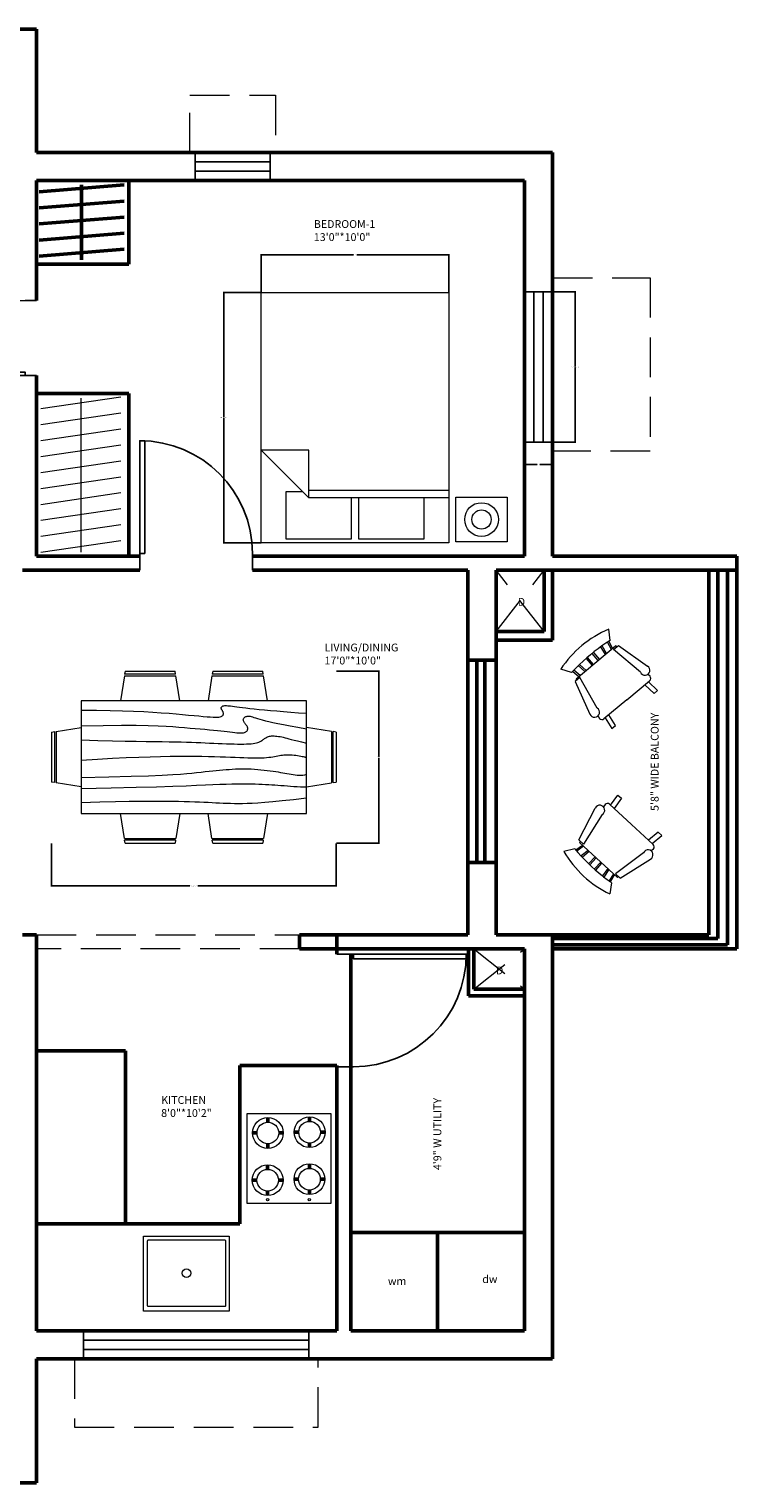
# Model space of a CAD drawing. Units: inches. Extents: x 291 to 2631, y 456 to 2623.
# Tile 19 of 22: x 2370 to 2596, y 1611 to 2076. Entities that reach past the tile are written whole.
import ezdxf

# ---------------------------------------------------------------- set-up
doc = ezdxf.new("R2010")
doc.units = ezdxf.units.IN
doc.linetypes.add('DASHED', pattern=[19.05, 12.7, -6.35])
for name, color, linetype, lineweight in [('A-ANNO-DIMS', 2, 'Continuous', 18), ('A-ANNO-TEXT', 3, 'Continuous', 25), ('A-AREA-IDEN', 7, 'Continuous', 25), ('A-DOOR', 3, 'Continuous', 25), ('A-FLOR-OVHD', 1, 'DASHED', 18), ('A-FURN', 8, 'Continuous', 18), ('A-GLAZ', 4, 'Continuous', 25), ('A-WALL', 7, 'Continuous', 50)]:
    doc.layers.add(name, color=color, linetype=linetype, lineweight=lineweight)
doc.styles.get("Standard").update_dxf_attribs({"font": 'arial.ttf'})
doc.dimstyles.get("Standard").update_dxf_attribs({"dimtxt": 0.18, "dimasz": 0.18, "dimexe": 0.18, "dimexo": 0.0625, "dimgap": 0.09, "dimtad": 0, "dimtih": 1, "dimtoh": 1, "dimdec": 4, "dimzin": 0, "dimdsep": 46, "dimtxsty": 'Standard', "dimcen": 0.09, "dimadec": 0, "dimazin": 0, "dimtfac": 1, "dimtdec": 4, "dimtofl": 0, "dimtmove": 0, "dimatfit": 3, "dimfxl": 1, "dimtolj": 1, "dimtzin": 0, "dimarcsym": 0})

# ---------------------------------------------------------------- blocks, each defined once
blk = doc.blocks.new('Bed - Queen')
for p, q in [((0, -80.00003), (0, 0)), ((0, 0), (59.99999, 0)), ((59.99999, 0), (59.99999, -80.00003)), ((7.99999, -1.2), (28.79998, -1.2)), ((7.99999, -14.4), (7.99999, -1.2)), ((28.79998, -1.2), (28.79998, -14.4)), ((31.19999, -1.2), (51.99999, -1.2)), ((31.19999, -14.4), (31.19999, -1.2)), ((51.99999, -1.2), (51.99999, -16.4)), ((0, -14.4), (44.8, -14.4)), ((44.8, -16.8), (0, -16.8)), ((59.99999, -29.6), (44.8, -14.4)), ((44.8, -14.4), (44.8, -29.6)), ((51.99999, -16.4), (46.79936, -16.4)), ((44.8, -29.6), (59.99999, -29.6)), ((59.99999, -80.00003), (0, -80.00003))]:
    blk.add_line(p, q)
blk = doc.blocks.new('Dining Set - 36 x 72 in.')
for p, q in [((-22.2343, 26.00059), (-23.4847, 17.99762)), ((-22.2304, 26), (-5.7608, 26)), ((-22, 27.5), (-22.1562, 26.50042)), ((-5.8416, 26.5), (-22.1534, 26.5)), ((-22, 27.5), (-6, 27.5)), ((-5.8437, 26.49966), (-6, 27.5)), ((-4.5152, 17.99762), (-5.7655, 25.99926)), ((5.7657, 26.00059), (4.5153, 17.99762)), ((5.7696, 26), (22.2392, 26)), ((6, 27.5), (5.8438, 26.50042)), ((22.1584, 26.5), (5.8466, 26.5)), ((6, 27.5), (22, 27.5)), ((22.1563, 26.49966), (22, 27.5)), ((23.4848, 17.99762), (22.2345, 25.99926)), ((36, 18), (-36, 18)), ((-36, 18), (-36, -18)), ((36, -18), (36, 18)), ((-44.0006, 8.23428), (-35.9976, 9.48474)), ((44.0006, 8.23428), (35.9976, 9.48474)), ((-45.5, 8), (-44.5004, 8.15617)), ((-45.5, 8), (-45.5, -8)), ((-44.5, -8.15843), (-44.5, 8.15338)), ((-44, 8.23041), (-44, -8.23915)), ((44, 8.23041), (44, -8.23915)), ((44.5, -8.15843), (44.5, 8.15338)), ((45.5, 8), (44.5005, 8.15617)), ((45.5, 8), (45.5, -8)), ((-44.4997, -8.15631), (-45.5, -8)), ((-35.9976, -9.48476), (-43.9993, -8.2345)), ((35.9976, -9.48476), (43.9993, -8.2345)), ((44.4997, -8.15631), (45.5, -8)), ((-36, -18), (36, -18)), ((-22.2343, -26.0006), (-23.4847, -17.99762)), ((-4.5152, -17.99762), (-5.7655, -25.99928)), ((5.7657, -26.0006), (4.5153, -17.99762)), ((23.4848, -17.99762), (22.2345, -25.99928)), ((-22.2304, -26), (-5.7608, -26)), ((-22, -27.5), (-22.1562, -26.50044)), ((-5.8416, -26.5), (-22.1534, -26.5)), ((-22, -27.5), (-6, -27.5)), ((-5.8437, -26.49967), (-6, -27.5)), ((5.7696, -26), (22.2392, -26)), ((6, -27.5), (5.8438, -26.50044)), ((22.1584, -26.5), (5.8466, -26.5)), ((6, -27.5), (22, -27.5)), ((22.1563, -26.49967), (22, -27.5))]:
    blk.add_line(p, q)
for points in [[(-36, 15), (-31.1772, 14.97754), (-26.8079, 14.91406), (-22.8538, 14.81543), (-19.276, 14.6875), (-16.0362, 14.53613), (-13.0957, 14.36718), (-10.4159, 14.18652), (-7.9583, 14), (-5.6904, 13.81315), (-3.6035, 13.63021), (-1.6954, 13.45508), (0.0365, 13.29166), (1.5945, 13.14388), (2.9811, 13.01562), (4.1988, 12.9108), (5.25, 12.83333), (6.1393, 12.78613), (6.8802, 12.76823), (7.4883, 12.77767), (7.9792, 12.8125), (8.3685, 12.87077), (8.6719, 12.95052), (8.9049, 13.0498), (9.0833, 13.16666), (9.2205, 13.29899), (9.3216, 13.44401), (9.3895, 13.59879), (9.4271, 13.76041), (9.4373, 13.92594), (9.4232, 14.09245), (9.3875, 14.257), (9.3333, 14.41666), (9.2638, 14.56917), (9.1836, 14.71484), (9.0975, 14.85465), (9.0104, 14.98958), (8.9272, 15.1206), (8.8529, 15.2487), (8.7922, 15.37483), (8.75, 15.5), (8.7305, 15.62467), (8.7344, 15.74739), (8.7617, 15.86621), (8.8125, 15.97916), (8.8867, 16.08431), (8.9844, 16.17968), (9.1055, 16.26334), (9.25, 16.33333), (9.4189, 16.38802), (9.6172, 16.42708), (9.8506, 16.45052), (10.125, 16.45833), (10.4463, 16.45052), (10.8203, 16.42708), (11.2529, 16.38802), (11.75, 16.33333), (12.3184, 16.26318), (12.9694, 16.17838), (13.7151, 16.07991), (14.5677, 15.96875), (15.5395, 15.84586), (16.6426, 15.71224), (17.8893, 15.56884), (19.2917, 15.41666), (20.859, 15.25667), (22.5879, 15.08984), (24.4721, 14.91715), (26.5052, 14.73958), (28.6809, 14.5581), (30.9929, 14.3737), (33.4347, 14.18733), (36, 14)], [(-36, 10), (-28.9766, 10.14274), (-23.1725, 10.20442), (-18.4241, 10.19775), (-14.5677, 10.13541), (-11.4399, 10.03011), (-8.877, 9.89453), (-6.7154, 9.74137), (-4.7917, 9.58333), (-2.9698, 9.43082), (-1.2246, 9.28515), (0.4415, 9.14534), (2.026, 9.01041), (3.5266, 8.87939), (4.9408, 8.7513), (6.266, 8.62516), (7.5, 8.5), (8.6411, 8.37549), (9.6914, 8.2539), (10.6538, 8.13818), (11.5312, 8.03125), (12.3267, 7.93603), (13.043, 7.85547), (13.6831, 7.79248), (14.25, 7.75), (14.7471, 7.7303), (15.1797, 7.73307), (15.5537, 7.75732), (15.875, 7.80208), (16.1494, 7.86637), (16.3828, 7.94922), (16.5811, 8.04964), (16.75, 8.16666), (16.8944, 8.29915), (17.0143, 8.44531), (17.1089, 8.60319), (17.1771, 8.77083), (17.218, 8.94629), (17.2305, 9.1276), (17.2137, 9.31282), (17.1667, 9.5), (17.0895, 9.6875), (16.987, 9.875), (16.8649, 10.0625), (16.7292, 10.25), (16.5856, 10.4375), (16.4401, 10.625), (16.2985, 10.8125), (16.1667, 11), (16.05, 11.18733), (15.9518, 11.3737), (15.8752, 11.5581), (15.8229, 11.73958), (15.798, 11.91715), (15.8034, 12.08984), (15.842, 12.25667), (15.9167, 12.41666), (16.0295, 12.56836), (16.1784, 12.70833), (16.3605, 12.83268), (16.5729, 12.9375), (16.8127, 13.01888), (17.0768, 13.07291), (17.3625, 13.0957), (17.6667, 13.08333), (17.9894, 13.03312), (18.3418, 12.94726), (18.7382, 12.82918), (19.1927, 12.68229), (19.7195, 12.51001), (20.3327, 12.31575), (21.0465, 12.10294), (21.875, 11.875), (22.8357, 11.63354), (23.959, 11.37304), (25.2786, 11.08618), (26.8282, 10.76562), (28.6414, 10.40405), (30.752, 9.99414), (33.1936, 9.52856), (36, 9)], [(-36, 5.5), (-30.7157, 5.3348), (-26.069, 5.20963), (-21.9946, 5.11767), (-18.4271, 5.05208), (-15.3009, 5.00602), (-12.5508, 4.97265), (-10.1112, 4.94515), (-7.9167, 4.91666), (-5.909, 4.88167), (-4.0586, 4.83984), (-2.3429, 4.79215), (-0.7396, 4.73958), (0.7739, 4.6831), (2.22, 4.6237), (3.6213, 4.56233), (5, 4.5), (6.373, 4.43782), (7.7344, 4.3776), (9.0723, 4.32129), (10.375, 4.27083), (11.6309, 4.22819), (12.8281, 4.19531), (13.9551, 4.17415), (15, 4.16666), (15.954, 4.17448), (16.819, 4.19791), (17.6001, 4.23698), (18.3021, 4.29166), (18.9299, 4.36198), (19.4883, 4.44791), (19.9823, 4.54948), (20.4167, 4.66666), (20.7969, 4.79899), (21.1302, 4.94401), (21.4245, 5.09879), (21.6875, 5.26041), (21.9271, 5.42594), (22.1511, 5.59245), (22.3672, 5.757), (22.5834, 5.91666), (22.8065, 6.06868), (23.0404, 6.21093), (23.2879, 6.34147), (23.5521, 6.45833), (23.8358, 6.55957), (24.142, 6.64323), (24.4735, 6.70735), (24.8334, 6.75), (25.2235, 6.76969), (25.642, 6.76692), (26.0858, 6.74267), (26.5521, 6.69791), (27.0379, 6.63362), (27.5404, 6.55078), (28.0565, 6.45036), (28.5834, 6.33333), (29.1242, 6.19987), (29.7071, 6.04687), (30.3661, 5.87044), (31.1354, 5.66666), (32.0493, 5.43164), (33.142, 5.16146), (34.4475, 4.85221), (36, 4.5)], [(-36, -1), (-30.7915, -0.6591), (-26.0195, -0.38216), (-21.6519, -0.16284), (-17.6563, 0.00521), (-14.0005, 0.12833), (-10.6523, 0.21289), (-7.5796, 0.26522), (-4.75, 0.29166), (-2.134, 0.29793), (0.2878, 0.28711), (2.5317, 0.26163), (4.6146, 0.22396), (6.5529, 0.17651), (8.3633, 0.12174), (10.0623, 0.06209), (11.6667, 0), (13.1899, -0.06201), (14.6341, -0.1211), (15.9982, -0.17432), (17.2813, -0.21875), (18.4823, -0.25147), (19.6003, -0.26953), (20.6343, -0.27002), (21.5834, -0.25), (22.4481, -0.20768), (23.2357, -0.14584), (23.9549, -0.06836), (24.6146, 0.02083), (25.2235, 0.11784), (25.7904, 0.21875), (26.3241, 0.31966), (26.8334, 0.41666), (27.3265, 0.50618), (27.8099, 0.58593), (28.2894, 0.65397), (28.7709, 0.70833), (29.2601, 0.74707), (29.763, 0.76823), (30.2855, 0.76985), (30.8334, 0.75), (31.4088, 0.70784), (31.9994, 0.64713), (32.589, 0.57275), (33.1615, 0.48958), (33.7008, 0.4025), (34.1908, 0.3164), (34.6153, 0.23616), (34.9584, 0.16666), (35.2099, 0.11165), (35.3848, 0.07031), (35.504, 0.04069), (35.5886, 0.02083), (35.6594, 0.00879), (35.7377, 0.0026), (35.8442, 0.00032), (36, 0)], [(-36, -6.5), (-27.1843, -6.31267), (-20.084, -6.1263), (-14.469, -5.9419), (-10.1094, -5.76042), (-6.7752, -5.58285), (-4.2363, -5.41016), (-2.2629, -5.24333), (-0.625, -5.08334), (0.8708, -4.93099), (2.2715, -4.78646), (3.5872, -4.64974), (4.8281, -4.52084), (6.0046, -4.39974), (7.127, -4.28646), (8.2053, -4.18099), (9.25, -4.08334), (10.2705, -3.99382), (11.2734, -3.91407), (12.2647, -3.84603), (13.25, -3.79167), (14.2354, -3.75293), (15.2266, -3.73177), (16.2295, -3.73015), (17.25, -3.75), (18.2912, -3.79248), (19.3451, -3.85547), (20.4009, -3.93604), (21.4479, -4.03125), (22.4754, -4.13819), (23.4727, -4.25391), (24.4289, -4.37549), (25.3334, -4.5), (26.1785, -4.62492), (26.9694, -4.74935), (27.7145, -4.87281), (28.4219, -4.99479), (29.1, -5.11483), (29.7572, -5.23242), (30.4016, -5.34709), (31.0417, -5.45834), (31.6837, -5.56437), (32.3262, -5.65821), (32.9658, -5.73153), (33.599, -5.77604), (34.2224, -5.78345), (34.8327, -5.74545), (35.4264, -5.65373), (36, -5.5)], [(-36, -10), (-26.4022, -9.81299), (-18.4675, -9.62891), (-11.9839, -9.45069), (-6.7396, -9.28125), (-2.5226, -9.12354), (0.8789, -8.98047), (3.6769, -8.85498), (6.0833, -8.75), (8.2767, -8.66765), (10.3021, -8.60677), (12.1712, -8.56543), (13.8958, -8.54167), (15.4876, -8.53353), (16.9583, -8.53907), (18.3197, -8.55632), (19.5834, -8.58334), (20.7616, -8.61841), (21.8685, -8.66081), (22.9188, -8.71004), (23.9271, -8.76563), (24.9081, -8.82707), (25.8763, -8.89388), (26.8465, -8.96558), (27.8334, -9.04167), (28.8474, -9.12118), (29.8828, -9.20117), (30.93, -9.27824), (31.9792, -9.34896), (33.0205, -9.40991), (34.0443, -9.45768), (35.0407, -9.48885), (36, -9.5)], [(-36, -14.5), (-30.0881, -14.33513), (-25.0332, -14.21224), (-20.7312, -14.12647), (-17.0781, -14.07292), (-13.97, -14.04671), (-11.3027, -14.04297), (-8.9724, -14.05681), (-6.875, -14.08334), (-4.9224, -14.11833), (-3.0905, -14.16016), (-1.3709, -14.20785), (0.2448, -14.26042), (1.7647, -14.3169), (3.1973, -14.3763), (4.5507, -14.43767), (5.8333, -14.5), (7.0554, -14.5621), (8.235, -14.62175), (9.3922, -14.67652), (10.5469, -14.72396), (11.7192, -14.76164), (12.929, -14.78711), (14.1965, -14.79794), (15.5417, -14.79167), (16.9933, -14.76424), (18.6152, -14.70508), (20.4804, -14.60197), (22.6615, -14.44271), (25.2312, -14.21509), (28.2624, -13.9069), (31.8277, -13.50594), (36, -13)]]:
    blk.add_lwpolyline(points)
blk = doc.blocks.new('Chair - Rocking')
for p, q in [((-8, -4.5), (-10, -1.5)), ((-7.5, -4.5), (-7, -7)), ((-6.5, -7), (-7.02225, -4.43)), ((-4.5, -7), (-4.96674, -4.19951)), ((-4, -7), (-4.40532, -4.16272)), ((-1.5, -4.05012), (-1.5, -7)), ((-1, -7), (-1, -4.05012)), ((1, -7), (1, -4.04655)), ((1.5, -4.05012), (1.5, -7)), ((4, -7), (4.40187, -4.18694)), ((4.5, -7), (4.96761, -4.19437)), ((6.5, -7), (7, -4.4057)), ((7.5, -4.5), (7, -7)), ((8, -4.5), (10, -1.5)), ((-9, -7.5), (-12, -18.49999)), ((-7, -7.5), (-9, -7.5)), ((-9, -18.49999), (-7, -7.5)), ((-8.23428, -6.99939), (-8.3093, -7.47958)), ((-8.23041, -7), (8.23915, -7)), ((7, -7.5), (9, -7.5)), ((9, -18.49999), (7, -7.5)), ((8.31071, -7.48854), (8.23449, -7.00073)), ((9, -7.5), (12, -18.49999)), ((-10.36644, -20.64523), (-10.5, -21.49999)), ((-9, -22.49999), (-9.5, -26.49999)), ((0, -22.49999), (-9.5, -22.49999)), ((-8, -26.49999), (-7.5, -22.49999)), ((0, -22.49999), (9.5, -22.49999)), ((8, -26.49999), (7.5, -22.49999)), ((9, -22.49999), (9.5, -26.49999)), ((10.5, -21.49999), (10.3575, -20.58798)), ((-9.5, -26.49999), (-8, -26.49999)), ((9.5, -26.49999), (8, -26.49999))]:
    blk.add_line(p, q)
for centre, radius, start, end in [((0, -34.08333), 34.08333, 72.93847, 107.0615), ((0, -68.25004), 64.25, 93.92211, 97.15267), ((0, -68.25004), 64.25, 82.84733, 93.92211), ((-10.5, -18.99999), 1.58114, 161.5651, 18.43495), ((10.5, -18.99999), 1.58114, 161.5651, 18.43495), ((-9.5, -21.49999), 1, 180, 270), ((9.5, -21.49999), 1, 270, 0)]:
    blk.add_arc(centre, radius, start, end)
blk = doc.blocks.new('*U2')
for p, q in [((0, 0), (0, -6)), ((40, 0), (40, -6))]:
    blk.add_line(p, q)
blk.add_lwpolyline([(0, 0), (0, 40), (1.75, 40), (1.75, 0)], close=True)
blk.add_arc((0, 0), 40, 0, 90)
blk = doc.blocks.new('WIN-1800')
for p, q in [((0, 9), (72, 9)), ((0, 0), (0, 9)), ((0, 6), (72, 6)), ((72, 9), (72, 0)), ((72, 3), (0, 3)), ((72, 0), (0, 0))]:
    blk.add_line(p, q)
blk = doc.blocks.new('WIN-1200')
for p, q in [((0, 0), (0, 48)), ((0, 48), (9, 48)), ((3, 0), (3, 48)), ((6, 48), (6, 0)), ((9, 48), (9, 0)), ((9, 0), (0, 0))]:
    blk.add_line(p, q)
blk = doc.blocks.new('WIN-600')
for p, q in [((24, 9), (0, 9)), ((0, 9), (0, 0)), ((24, 6), (0, 6)), ((24, 0), (24, 9)), ((0, 3), (24, 3)), ((0, 0), (24, 0))]:
    blk.add_line(p, q)
blk = doc.blocks.new('*D24')
at = {"layer": 'A-ANNO-DIMS', "color": 0, "lineweight": -2, "transparency": 16777216}
for p, q in [((2537.27, 1991.61), (2544.59, 1991.61)), ((2544.41, 1991.43), (2544.41, 1967.79)), ((2544.41, 1943.79), (2544.41, 1967.43)), ((2537.27, 1943.61), (2544.59, 1943.61))]:
    blk.add_line(p, q, dxfattribs=at)
at = {"layer": 'A-ANNO-DIMS', "color": 0, "transparency": 16777216}
for points in [[(2544.38, 1991.43), (2544.44, 1991.43), (2544.41, 1991.61)], [(2544.38, 1943.79), (2544.44, 1943.79), (2544.41, 1943.61)]]:
    blk.add_solid(points, dxfattribs=at)
at = {"layer": 'DEFPOINTS', "color": 0, "transparency": 16777216}
for p in [(2537.21, 1991.61), (2544.41, 1991.61), (2537.21, 1943.61)]:
    blk.add_point(p, dxfattribs=at)
at = {"layer": 'A-ANNO-DIMS', "color": 0, "transparency": 16777216, "insert": (2544.41, 1967.61), "char_height": 0.18, "attachment_point": 5}
blk.add_mtext('\\A1;WINDOW W1200 48 TYP.', dxfattribs=at)
blk = doc.blocks.new('*D25')
at = {"layer": 'A-ANNO-DIMS', "color": 0, "lineweight": -2, "transparency": 16777216}
for p, q in [((2528.21, 1943.55), (2528.21, 1936.23)), ((2537.21, 1943.55), (2537.21, 1936.23)), ((2528.39, 1936.41), (2532.25, 1936.41)), ((2537.03, 1936.41), (2533.16, 1936.41))]:
    blk.add_line(p, q, dxfattribs=at)
at = {"layer": 'A-ANNO-DIMS', "color": 0, "transparency": 16777216}
for points in [[(2528.39, 1936.44), (2528.39, 1936.38), (2528.21, 1936.41)], [(2537.03, 1936.44), (2537.03, 1936.38), (2537.21, 1936.41)]]:
    blk.add_solid(points, dxfattribs=at)
at = {"layer": 'DEFPOINTS', "color": 0, "transparency": 16777216}
for p in [(2528.21, 1943.61), (2537.21, 1943.61), (2537.21, 1936.41)]:
    blk.add_point(p, dxfattribs=at)
at = {"layer": 'A-ANNO-DIMS', "color": 0, "transparency": 16777216, "insert": (2532.71, 1936.41), "char_height": 0.18, "attachment_point": 5}
blk.add_mtext('\\A1;9 TYP.', dxfattribs=at)
blk = doc.blocks.new('*D28')
at = {"layer": 'A-ANNO-DIMS', "color": 0, "lineweight": -2, "transparency": 16777216}
for p, q in [((2443.99, 1991.43), (2431.88, 1991.43)), ((2432.06, 1991.25), (2432.06, 1951.62)), ((2432.06, 1911.61), (2432.06, 1951.24)), ((2443.99, 1911.43), (2431.88, 1911.43))]:
    blk.add_line(p, q, dxfattribs=at)
at = {"layer": 'A-ANNO-DIMS', "color": 0, "transparency": 16777216}
for points in [[(2432.03, 1991.25), (2432.09, 1991.25), (2432.06, 1991.43)], [(2432.03, 1911.61), (2432.09, 1911.61), (2432.06, 1911.43)]]:
    blk.add_solid(points, dxfattribs=at)
at = {"layer": 'DEFPOINTS', "color": 0, "transparency": 16777216}
for p in [(2444.06, 1991.43), (2432.06, 1911.43), (2444.06, 1911.43)]:
    blk.add_point(p, dxfattribs=at)
at = {"layer": 'A-ANNO-DIMS', "color": 0, "transparency": 16777216, "insert": (2432.06, 1951.43), "char_height": 0.18, "attachment_point": 5}
blk.add_mtext('\\A1;QUEEN BED 80 TYP.', dxfattribs=at)
blk = doc.blocks.new('*D29')
at = {"layer": 'A-ANNO-DIMS', "color": 0, "lineweight": -2, "transparency": 16777216}
for p, q in [((2444.06, 1991.49), (2444.06, 2003.61)), ((2444.24, 2003.43), (2473.53, 2003.43)), ((2503.88, 2003.43), (2474.58, 2003.43)), ((2504.06, 1991.49), (2504.06, 2003.61))]:
    blk.add_line(p, q, dxfattribs=at)
at = {"layer": 'A-ANNO-DIMS', "color": 0, "transparency": 16777216}
for points in [[(2444.24, 2003.46), (2444.24, 2003.4), (2444.06, 2003.43)], [(2503.88, 2003.46), (2503.88, 2003.4), (2504.06, 2003.43)]]:
    blk.add_solid(points, dxfattribs=at)
at = {"layer": 'DEFPOINTS', "color": 0, "transparency": 16777216}
for p in [(2444.06, 2003.43), (2444.06, 1991.43), (2504.06, 1991.43)]:
    blk.add_point(p, dxfattribs=at)
at = {"layer": 'A-ANNO-DIMS', "color": 0, "transparency": 16777216, "insert": (2474.06, 2003.43), "char_height": 0.18, "attachment_point": 5}
blk.add_mtext('\\A1;60 TYP.', dxfattribs=at)
blk = doc.blocks.new('*D46')
at = {"layer": 'A-ANNO-DIMS', "color": 0, "lineweight": -2, "transparency": 16777216}
for p, q in [((2377.04, 1815.38), (2377.04, 1801.62)), ((2468.04, 1815.38), (2468.04, 1801.62)), ((2377.22, 1801.8), (2421.26, 1801.8)), ((2467.86, 1801.8), (2423.82, 1801.8))]:
    blk.add_line(p, q, dxfattribs=at)
at = {"layer": 'A-ANNO-DIMS', "color": 0, "transparency": 16777216}
for points in [[(2377.22, 1801.83), (2377.22, 1801.77), (2377.04, 1801.8)], [(2467.86, 1801.83), (2467.86, 1801.77), (2468.04, 1801.8)]]:
    blk.add_solid(points, dxfattribs=at)
at = {"layer": 'DEFPOINTS', "color": 0, "transparency": 16777216}
for p in [(2377.04, 1815.45), (2468.04, 1815.45), (2468.04, 1801.8)]:
    blk.add_point(p, dxfattribs=at)
at = {"layer": 'A-ANNO-DIMS', "color": 0, "transparency": 16777216, "insert": (2422.54, 1801.8), "char_height": 0.18, "attachment_point": 5}
blk.add_mtext('\\A1;DINING SET 91 TYP.', dxfattribs=at)
blk = doc.blocks.new('*D47')
at = {"layer": 'A-ANNO-DIMS', "color": 0, "lineweight": -2, "transparency": 16777216}
for p, q in [((2468.1, 1870.45), (2481.87, 1870.45)), ((2481.69, 1870.27), (2481.69, 1843.13)), ((2481.69, 1815.63), (2481.69, 1842.77)), ((2468.1, 1815.45), (2481.87, 1815.45))]:
    blk.add_line(p, q, dxfattribs=at)
at = {"layer": 'A-ANNO-DIMS', "color": 0, "transparency": 16777216}
for points in [[(2481.66, 1870.27), (2481.72, 1870.27), (2481.69, 1870.45)], [(2481.66, 1815.63), (2481.72, 1815.63), (2481.69, 1815.45)]]:
    blk.add_solid(points, dxfattribs=at)
at = {"layer": 'DEFPOINTS', "color": 0, "transparency": 16777216}
for p in [(2468.04, 1870.45), (2481.69, 1870.45), (2468.04, 1815.45)]:
    blk.add_point(p, dxfattribs=at)
at = {"layer": 'A-ANNO-DIMS', "color": 0, "transparency": 16777216, "insert": (2481.69, 1842.95), "char_height": 0.18, "attachment_point": 5}
blk.add_mtext('\\A1;55 TYP.', dxfattribs=at)

msp = doc.modelspace()

# ---------------------------------------------------------------- linework, layer by layer
at = {"layer": 'A-FLOR-OVHD'}
for p, q in [((2421.24, 2036.14), (2421.24, 2054.42)), ((2421.24, 2054.42), (2448.64, 2054.42)), ((2448.64, 2054.42), (2448.64, 2036.14)), ((2537.21, 1996.12), (2568.43, 1996.12)), ((2568.43, 1996.12), (2568.43, 1940.67)), ((2568.43, 1940.67), (2537.21, 1940.67)), ((2519.14, 1883.06), (2534.51, 1902.64)), ((2534.51, 1883.06), (2519.14, 1902.64)), ((2372.21, 1786.14), (2456.28, 1786.14)), ((2456.28, 1781.64), (2372.21, 1781.64)), ((2512, 1781.64), (2528.21, 1768.81)), ((2512, 1768.81), (2528.21, 1781.64)), ((2384.4, 1650.64), (2384.4, 1628.9)), ((2462.3, 1628.9), (2462.3, 1650.64)), ((2384.4, 1628.9), (2462.3, 1628.9))]:
    msp.add_line(p, q, dxfattribs=at)
at = {"layer": 'A-FURN'}
for p, q in [((2373.6, 1954.3), (2399.2, 1958.03)), ((2386.4, 1957.68), (2386.4, 1908.48)), ((2373.6, 1949.2), (2399.2, 1952.94)), ((2373.6, 1944.1), (2399.2, 1947.84)), ((2373.6, 1939.01), (2399.2, 1942.74)), ((2373.6, 1933.91), (2399.2, 1937.64)), ((2373.6, 1928.81), (2399.2, 1932.54)), ((2373.6, 1923.71), (2399.2, 1927.45)), ((2373.6, 1918.61), (2399.2, 1922.35)), ((2373.6, 1913.52), (2399.2, 1917.25)), ((2373.6, 1908.42), (2399.2, 1912.15))]:
    msp.add_line(p, q, dxfattribs=at)
for points in [[(2506.25, 1926.01), (2522.73, 1926.01), (2522.73, 1911.71), (2506.25, 1911.71)], [(2439.58, 1729.09), (2466.29, 1729.09), (2466.29, 1700.32), (2439.58, 1700.32)], [(2406.4, 1689.84), (2433.84, 1689.84), (2433.84, 1665.94), (2406.4, 1665.94)]]:
    msp.add_lwpolyline(points, close=True, dxfattribs=at)
msp.add_lwpolyline([(2408.04, 1688.73), (2432.34, 1688.73, -0.414214), (2432.64, 1688.43), (2432.64, 1667.66, -0.414214), (2432.34, 1667.36), (2408.04, 1667.36, -0.414214), (2407.74, 1667.66), (2407.74, 1688.43, -0.414214)], format="xyb", close=True, dxfattribs=at)
for centre, radius in [((2514.49, 1918.86), 5.39), ((2514.49, 1918.86), 3.08), ((2446.18, 1722.85), 4.92), ((2446.18, 1722.85), 3.46), ((2459.53, 1723.1), 4.92), ((2459.53, 1723.1), 3.46), ((2446.12, 1707.77), 4.92), ((2446.12, 1707.77), 3.46), ((2459.47, 1708.09), 4.92), ((2459.47, 1708.09), 3.46), ((2446.08, 1701.54), 0.363), ((2459.43, 1701.55), 0.363), ((2420.19, 1678.04), 1.36)]:
    msp.add_circle(centre, radius, dxfattribs=at)
at = {"layer": 'A-WALL'}
for p, q in [((2303.21, 2075.57), (2372.21, 2075.57)), ((2372.21, 2075.57), (2372.21, 2036.14)), ((2372.21, 2036.14), (2521.26, 2036.14)), ((2537.21, 2036.14), (2521.26, 2036.14)), ((2537.21, 2027.14), (2537.21, 2036.14)), ((2372.21, 2027.14), (2372.21, 1988.89)), ((2372.21, 2027.14), (2372.21, 1988.89)), ((2372.21, 2027.14), (2521.26, 2027.14)), ((2373.04, 2023.54), (2400.26, 2025.76)), ((2386.65, 2025.83), (2386.65, 2001.89)), ((2401.79, 2000.49), (2401.79, 2027.14)), ((2521.26, 2027.14), (2528.21, 2027.14)), ((2528.21, 2027.14), (2528.21, 1907.14)), ((2537.21, 2027.14), (2537.21, 1907.14)), ((2373.04, 2018.42), (2400.26, 2020.64)), ((2373.04, 2013.3), (2400.26, 2015.52)), ((2373.04, 2008.17), (2400.26, 2010.39)), ((2373.04, 2003.05), (2400.26, 2005.27)), ((2372.21, 2000.49), (2401.79, 2000.49)), ((2372.21, 1964.89), (2372.21, 1907.14)), ((2372.21, 1964.89), (2372.21, 1907.14)), ((2372.21, 1959.17), (2401.79, 1959.17)), ((2401.79, 1959.17), (2401.79, 1907.14)), ((2372.21, 1907.14), (2405.25, 1907.14)), ((2441.25, 1907.14), (2528.21, 1907.14)), ((2537.21, 1907.14), (2596.14, 1907.14)), ((2596.14, 1907.14), (2596.14, 1781.64)), ((2367.71, 1902.64), (2405.25, 1902.64)), ((2441.25, 1902.64), (2510.14, 1902.64)), ((2510.14, 1902.64), (2510.14, 1786.14)), ((2519.14, 1902.64), (2519.14, 1786.14)), ((2519.14, 1902.64), (2537.21, 1902.64)), ((2534.51, 1883.06), (2534.51, 1902.64)), ((2537.21, 1902.64), (2587.14, 1902.64)), ((2537.21, 1880.36), (2537.21, 1902.64)), ((2587.14, 1902.64), (2587.14, 1786.14)), ((2587.14, 1902.64), (2596.14, 1902.64)), ((2590.07, 1902.64), (2590.07, 1785.04)), ((2593.07, 1902.64), (2593.07, 1782.94)), ((2519.14, 1883.06), (2534.51, 1883.06)), ((2519.14, 1880.36), (2537.21, 1880.36)), ((2510.14, 1873.98), (2519.14, 1873.98)), ((2513.01, 1873.98), (2513.01, 1809.26)), ((2515.57, 1873.98), (2515.57, 1809.26)), ((2510.14, 1809.26), (2519.14, 1809.26)), ((2372.21, 1786.14), (2367.71, 1786.14)), ((2372.21, 1786.14), (2372.21, 1659.64)), ((2456.28, 1786.14), (2510.14, 1786.14)), ((2456.28, 1786.14), (2456.28, 1781.64)), ((2468.21, 1786.14), (2468.21, 1780.04)), ((2519.14, 1786.14), (2537.21, 1786.14)), ((2537.21, 1786.14), (2537.21, 1650.64)), ((2537.21, 1786.14), (2587.14, 1786.14)), ((2590.07, 1785.04), (2537.21, 1785.04)), ((2456.28, 1781.64), (2528.21, 1781.64)), ((2472.71, 1780.04), (2472.71, 1659.64)), ((2510.28, 1781.64), (2510.28, 1766.69)), ((2512, 1781.64), (2512, 1768.81)), ((2528.21, 1781.64), (2528.21, 1659.64)), ((2593.07, 1782.94), (2537.21, 1782.94)), ((2537.21, 1781.64), (2596.14, 1781.64)), ((2510.28, 1766.69), (2528.21, 1766.69)), ((2512, 1768.81), (2528.21, 1768.81)), ((2371.98, 1749.09), (2400.7, 1749.09)), ((2400.7, 1749.09), (2400.7, 1693.87)), ((2437.25, 1693.87), (2437.25, 1744.38)), ((2437.25, 1744.38), (2440.94, 1744.38)), ((2440.94, 1744.38), (2468.21, 1744.38)), ((2468.21, 1744.38), (2468.21, 1659.64)), ((2446.18, 1726.31), (2446.18, 1727.77)), ((2459.53, 1726.56), (2459.53, 1728.02)), ((2441.26, 1722.85), (2442.72, 1722.85)), ((2446.18, 1719.39), (2446.18, 1717.93)), ((2449.65, 1722.85), (2451.1, 1722.85)), ((2454.61, 1723.1), (2456.06, 1723.1)), ((2459.53, 1719.63), (2459.53, 1718.18)), ((2462.99, 1723.1), (2464.45, 1723.1)), ((2446.12, 1711.23), (2446.12, 1712.69)), ((2459.47, 1711.55), (2459.47, 1713.01)), ((2441.2, 1707.77), (2442.66, 1707.77)), ((2449.58, 1707.77), (2451.04, 1707.77)), ((2454.55, 1708.09), (2456, 1708.09)), ((2462.93, 1708.09), (2464.39, 1708.09)), ((2446.12, 1704.31), (2446.12, 1702.85)), ((2459.47, 1704.63), (2459.47, 1703.17)), ((2400.7, 1693.87), (2372.21, 1693.87)), ((2400.7, 1693.87), (2437.25, 1693.87)), ((2472.71, 1691.05), (2528.21, 1691.05)), ((2500.46, 1691.05), (2500.46, 1659.64)), ((2372.21, 1659.64), (2468.21, 1659.64)), ((2472.71, 1659.64), (2528.21, 1659.64)), ((2372.21, 1650.64), (2537.21, 1650.64)), ((2372.21, 1611.04), (2372.21, 1650.64)), ((2303.21, 1611.04), (2372.21, 1611.04))]:
    msp.add_line(p, q, dxfattribs=at)

# ---------------------------------------------------------------- block references
at = {"layer": 'A-DOOR'}
for p, xscale, yscale, zscale, rotation in [((2368.61, 1964.89), 0.6, 0.6, 0.6, 90.00000000000003), ((2473.61, 1780.04), 0.9, 0.9, 0.9, 270)]:
    msp.add_blockref('*U2', p, dxfattribs=dict(at, xscale=xscale, yscale=yscale, zscale=zscale, rotation=rotation))
at = {"layer": 'A-DOOR', "xscale": 0.9, "yscale": 0.9, "zscale": 0.9}
msp.add_blockref('*U2', (2405.25, 1908.04), dxfattribs=at)
at = {"layer": 'A-FURN'}
for name, p, rotation in [('Bed - Queen', (2504.06, 1911.43), 180), ('Chair - Rocking', (2546.54, 1878.58), 39.75679378516137), ('Chair - Rocking', (2547.13, 1804.91), 137.3178093086548)]:
    msp.add_blockref(name, p, dxfattribs=dict(at, rotation=rotation))
msp.add_blockref('Dining Set - 36 x 72 in.', (2422.54, 1842.95), dxfattribs=at)
at = {"layer": 'A-GLAZ', "rotation": 180}
msp.add_blockref('WIN-600', (2446.96, 2036.14), dxfattribs=at)
at = {"layer": 'A-GLAZ'}
for name, p in [('WIN-1200', (2528.21, 1943.61)), ('WIN-1800', (2387.26, 1650.64))]:
    msp.add_blockref(name, p, dxfattribs=at)

# ---------------------------------------------------------------- texts
at = {"layer": 'A-ANNO-TEXT', "char_height": 2.5, "attachment_point": 1}
for s, width, insert in [('D', 1.7284, (2526.07, 1893.81)), ('D', 2.5248, (2519.09, 1776.03)), ('dw', 14.3674, (2514.72, 1677.41)), ('wm', 19.2983, (2484.57, 1676.78))]:
    msp.add_mtext_dynamic_manual_height_columns(s, width=width, gutter_width=12.5, heights=[0], dxfattribs=dict(at, insert=insert))
at = {"layer": 'A-AREA-IDEN', "char_height": 2.5, "attachment_point": 1}
for s, width, insert in [('BEDROOM-1\\P13\'0"*10\'0"', 79.5755, (2460.88, 2014.53)), ('LIVING/DINING\\P17\'0"*10\'0"', 49.1615, (2464.29, 1879.22)), ('KITCHEN\\P8\'0"*10\'2"', 31.4504, (2412.07, 1734.64))]:
    msp.add_mtext_dynamic_manual_height_columns(s, width=width, gutter_width=12.5, heights=[0], dxfattribs=dict(at, insert=insert))
at = {"layer": 'A-AREA-IDEN', "char_height": 2.5, "attachment_point": 1, "rotation": 90}
for s, width, insert in [('5\'8" WIDE BALCONY', 47.5655, (2568.6, 1825.75)), ('4\'9" W UTILITY', 41.3064, (2499.13, 1710.99))]:
    msp.add_mtext_dynamic_manual_height_columns(s, width=width, gutter_width=12.5, heights=[0], dxfattribs=dict(at, insert=insert))

# ---------------------------------------------------------------- dimensions: what is measured, and where the dimension line sits
at = {"layer": 'A-ANNO-DIMS'}
for base, p1, p2, angle, text, picture, middle in [((2444.06, 2003.43), (2504.06, 1991.43), (2444.06, 1991.43), 180, '<> TYP.', '*D29', (2474.06, 2003.43)), ((2432.06, 1911.43), (2444.06, 1991.43), (2444.06, 1911.43), 270, 'QUEEN BED <> TYP.', '*D28', (2432.06, 1951.43)), ((2544.41, 1991.61), (2537.21, 1943.61), (2537.21, 1991.61), 90, 'WINDOW W1200 <> TYP.', '*D24', (2544.41, 1967.61)), ((2481.69, 1870.45), (2468.04, 1815.45), (2468.04, 1870.45), 90, '<> TYP.', '*D47', (2481.69, 1842.95))]:
    dim = msp.add_linear_dim(base=base, p1=p1, p2=p2, angle=angle, text=text, dimstyle='Standard', override={"dimdec": 0, "dimlfac": 1, "dimrnd": 0, "dimzin": 0, "dimdsep": 46, "dimlunit": 2}, dxfattribs=at)
    dim.commit()
    dim.dimension.update_dxf_attribs({"geometry": picture, "text_midpoint": middle})
for base, p1, p2, text, picture, middle in [((2537.21, 1936.41), (2528.21, 1943.61), (2537.21, 1943.61), '<> TYP.', '*D25', (2532.71, 1936.41)), ((2468.04, 1801.8), (2377.04, 1815.45), (2468.04, 1815.45), 'DINING SET <> TYP.', '*D46', (2422.54, 1801.8))]:
    dim = msp.add_linear_dim(base=base, p1=p1, p2=p2, text=text, dimstyle='Standard', override={"dimdec": 0, "dimlfac": 1, "dimrnd": 0, "dimzin": 0, "dimdsep": 46, "dimlunit": 2}, dxfattribs=at)
    dim.commit()
    dim.dimension.update_dxf_attribs({"geometry": picture, "text_midpoint": middle})

doc.saveas('drawing.dxf')
